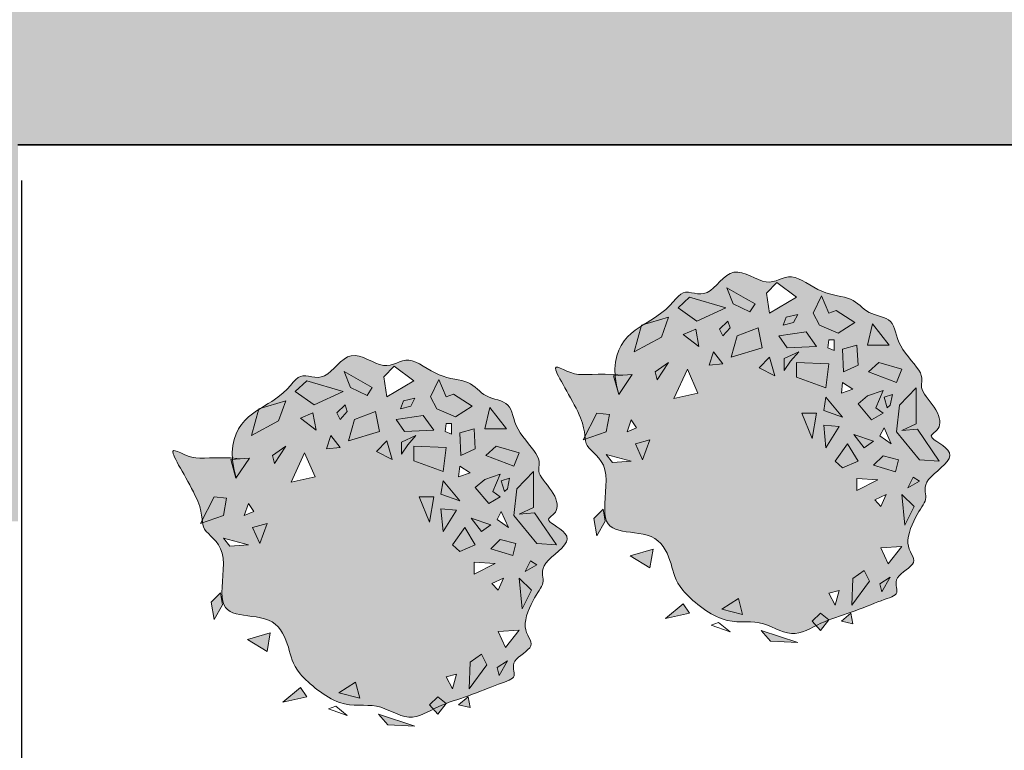
# Model space of a CAD drawing. Units: metres. Extents: x 4298.5 to 4325.2, y 2075 to 2095.8.
# Tile 30 of 35: x 4320.314 to 4321.936, y 2083.561 to 2084.765. Entities that reach past the tile are written whole.
import ezdxf

# ---------------------------------------------------------------- set-up
doc = ezdxf.new("R2010")
doc.units = ezdxf.units.M
for name, color, linetype, lineweight in [('A-ANNO-DIMS', 2, 'Continuous', 18), ('A-WALL', 7, 'Continuous', 35), ('A-WALL-PATT', 252, 'Continuous', 13), ('L-PLNT', 94, 'Continuous', 13)]:
    doc.layers.add(name, color=color, linetype=linetype, lineweight=lineweight)
doc.layers.add('L-PLNT-PATT', color=116, linetype='Continuous', lineweight=13, true_color=0x13823e)
doc.styles.get("Standard").update_dxf_attribs({"font": 'arial.ttf'})
doc.dimstyles.get("Standard").update_dxf_attribs({"dimtxt": 0.18, "dimasz": 0.18, "dimexe": 0.18, "dimexo": 0.0625, "dimgap": 0.09, "dimtad": 0, "dimtih": 1, "dimtoh": 1, "dimdec": 4, "dimzin": 0, "dimdsep": 46, "dimtxsty": 'Standard', "dimcen": 0.09, "dimadec": 0, "dimazin": 0, "dimtfac": 1, "dimtdec": 4, "dimtofl": 0, "dimtmove": 0, "dimatfit": 3, "dimfxl": 1, "dimtolj": 1, "dimtzin": 0, "dimarcsym": 0})

# ---------------------------------------------------------------- blocks, each defined once
blk = doc.blocks.new('*U9')
for points in [[(-2.003, 11.656), (-1.598, 10.618), (-0.518, 10.099), (-0.181, 10.618), (-0.788, 10.964)], [(1.237, 12.003), (0.562, 11.31), (0.764, 10.013), (2.519, 11.051)], [(-4.432, 11.051), (-5.175, 10.359), (-3.96, 9.493), (-2.07, 10.359)], [(4.139, 11.137), (3.599, 10.013), (4.004, 9.234), (5.218, 8.715), (6.298, 9.407), (5.083, 10.186), (4.611, 10.013)], [(-5.782, 9.753), (-7.537, 9.234), (-8.009, 7.504), (-6.255, 8.455)], [(2.586, 9.926), (1.844, 9.753), (1.642, 9.234), (2.316, 9.407)], [(-4.837, 8.628), (-3.825, 7.85), (-4.027, 8.974)], [(-1.935, 9.493), (-2.475, 8.974), (-2.273, 8.542), (-1.8, 9.061)], [(0.022, 9.061), (-1.328, 8.542), (-1.733, 7.157), (0.292, 7.763)], [(7.446, 9.32), (7.108, 7.936), (8.525, 7.936)], [(1.372, 8.542), (3.126, 8.801), (3.801, 7.85), (1.912, 7.763)], [(4.611, 8.282), (4.544, 7.763), (4.949, 7.59), (4.949, 8.282)], [(6.433, 7.936), (5.488, 7.676), (5.556, 6.206), (6.501, 6.638)], [(-2.88, 7.504), (-3.15, 6.638), (-2.273, 6.725)], [(0.764, 7.157), (0.089, 6.465), (1.102, 5.946)], [(1.709, 6.292), (1.709, 7.071), (2.654, 7.504), (2.114, 6.898)], [(-5.782, 6.811), (-6.659, 6.206), (-6.524, 5.687)], [(2.519, 6.811), (2.519, 5.86), (4.409, 5.167), (4.611, 6.725)], [(7.851, 6.811), (7.176, 6.206), (8.998, 5.514), (9.335, 6.379)], [(-8.144, 6.033), (-9.359, 5.946), (-9.022, 4.735)], [(-4.567, 6.379), (-5.445, 4.475), (-3.892, 4.821)], [(5.488, 5.514), (5.421, 4.821), (6.163, 5.081)], [(10.28, 5.167), (9.2, 4.043), (8.998, 2.312), (10.482, 0.495), (11.765, 0.409), (10.348, 2.485), (9.335, 2.399), (10.28, 2.831)], [(4.409, 4.562), (4.274, 3.697), (5.488, 3.264)], [(8.12, 4.994), (7.108, 4.648), (6.501, 4.129), (7.378, 3.091), (8.12, 3.524), (7.648, 3.87)], [(8.728, 4.735), (8.188, 4.562), (8.39, 3.87), (8.593, 4.043)], [(-11.316, 1.793), (-9.831, 2.312), (-9.629, 3.437), (-10.439, 3.524)], [(3.531, 1.88), (2.856, 3.524), (3.801, 3.524)], [(-8.212, 3.091), (-8.482, 2.312), (-7.874, 2.572)], [(4.274, 2.745), (5.286, 2.658), (4.409, 1.274)], [(8.188, 2.572), (7.918, 2.053), (8.66, 1.534)], [(7.513, 1.707), (6.906, 1.274), (6.231, 2.139)], [(-6.997, 1.793), (-7.942, 1.534), (-7.469, 0.495)], [(5.826, 1.534), (5.016, 0.409), (5.488, -0.024), (6.501, 0.409)], [(-8.212, 0.409), (-9.426, 0.322), (-9.831, 0.841)], [(8.12, 0.755), (7.513, 0.149), (8.93, -0.283), (9.133, 0.495)], [(10.078, -0.629), (9.74, -1.322), (10.482, -0.889)], [(7.783, -0.803), (6.433, -1.495), (6.433, -0.716)], [(8.323, -1.754), (7.985, -2.533), (7.581, -2.1)], [(9.335, -1.754), (9.538, -3.744), (10.145, -2.533)], [(-10.034, -2.706), (-10.641, -3.312), (-10.439, -4.436), (-9.899, -3.485)], [(-8.279, -5.734), (-6.794, -5.302), (-6.997, -6.513)], [(9.335, -5.129), (8.458, -6.253), (7.985, -5.215)], [(6.096, -8.935), (6.163, -7.205), (6.906, -6.686), (7.243, -7.378)], [(8.053, -8.07), (8.593, -7.118), (7.918, -7.551)], [(5.286, -7.984), (4.611, -8.157), (5.016, -8.935)], [(-4.837, -8.849), (-4.432, -9.454), (-5.985, -9.801)], [(-2.34, -9.195), (-1.26, -8.503), (-0.99, -9.541)], [(4.071, -9.454), (3.531, -9.974), (4.071, -10.579), (4.611, -9.887)], [(6.028, -9.454), (5.421, -9.974), (6.163, -10.147)], [(-2.543, -10.06), (-3.015, -10.233), (-1.8, -10.666)], [(0.224, -10.579), (0.832, -11.272), (2.586, -11.358)]]:
    blk.add_lwpolyline(points, close=True)
blk = doc.blocks.new('*D47')
at = {"layer": 'A-ANNO-DIMS', "color": 0, "lineweight": -2, "transparency": 16777216}
for p, q in [((4300.4306, 2084.4956), (4300.4306, 2074.9896)), ((4322.8106, 2084.4956), (4322.8106, 2074.9896)), ((4300.6106, 2075.1696), (4311.2252, 2075.1696)), ((4322.6306, 2075.1696), (4312.016, 2075.1696))]:
    blk.add_line(p, q, dxfattribs=at)
at = {"layer": 'A-ANNO-DIMS', "color": 0, "transparency": 16777216}
for points in [[(4300.6106, 2075.1996), (4300.6106, 2075.1396), (4300.4306, 2075.1696)], [(4322.6306, 2075.1996), (4322.6306, 2075.1396), (4322.8106, 2075.1696)]]:
    blk.add_solid(points, dxfattribs=at)
at = {"layer": 'Defpoints', "color": 0, "transparency": 16777216}
for p in [(4300.4306, 2084.5581), (4322.8106, 2084.5581), (4322.8106, 2075.1696)]:
    blk.add_point(p, dxfattribs=at)
at = {"layer": 'A-ANNO-DIMS', "color": 0, "transparency": 16777216, "insert": (4311.6206, 2075.1696), "char_height": 0.18, "attachment_point": 5}
blk.add_mtext('\\A1;22.38', dxfattribs=at)
blk = doc.blocks.new('*D48')
at = {"layer": 'A-ANNO-DIMS', "color": 0, "lineweight": -2, "transparency": 16777216}
for p, q in [((4310.1831, 2094.4781), (4324.7671, 2094.4781)), ((4324.5871, 2094.2981), (4324.5871, 2085.585)), ((4324.5871, 2076.5081), (4324.5871, 2085.2212)), ((4316.8731, 2076.3281), (4324.7671, 2076.3281))]:
    blk.add_line(p, q, dxfattribs=at)
at = {"layer": 'A-ANNO-DIMS', "color": 0, "transparency": 16777216}
for points in [[(4324.5571, 2094.2981), (4324.6171, 2094.2981), (4324.5871, 2094.4781)], [(4324.5571, 2076.5081), (4324.6171, 2076.5081), (4324.5871, 2076.3281)]]:
    blk.add_solid(points, dxfattribs=at)
at = {"layer": 'Defpoints', "color": 0, "transparency": 16777216}
for p in [(4310.1206, 2094.4781), (4316.8106, 2076.3281), (4324.5871, 2076.3281)]:
    blk.add_point(p, dxfattribs=at)
at = {"layer": 'A-ANNO-DIMS', "color": 0, "transparency": 16777216, "insert": (4324.5871, 2085.4031), "char_height": 0.18, "attachment_point": 5}
blk.add_mtext('\\A1;18.15', dxfattribs=at)
blk = doc.blocks.new('*D55')
at = {"layer": 'A-ANNO-DIMS', "color": 0, "lineweight": -2, "transparency": 16777216}
for p, q in [((4320.3167, 2084.4996), (4320.3167, 2074.9896)), ((4322.8106, 2084.4956), (4322.8106, 2074.9896)), ((4320.4967, 2075.1696), (4321.1688, 2075.1696)), ((4322.6306, 2075.1696), (4321.9585, 2075.1696))]:
    blk.add_line(p, q, dxfattribs=at)
at = {"layer": 'A-ANNO-DIMS', "color": 0, "transparency": 16777216}
for points in [[(4320.4967, 2075.1996), (4320.4967, 2075.1396), (4320.3167, 2075.1696)], [(4322.6306, 2075.1996), (4322.6306, 2075.1396), (4322.8106, 2075.1696)]]:
    blk.add_solid(points, dxfattribs=at)
at = {"layer": 'Defpoints', "color": 0, "transparency": 16777216}
for p in [(4320.3167, 2084.5621), (4322.8106, 2084.5581), (4322.8106, 2075.1696)]:
    blk.add_point(p, dxfattribs=at)
at = {"layer": 'A-ANNO-DIMS', "color": 0, "transparency": 16777216, "insert": (4321.5636, 2075.1696), "char_height": 0.18, "attachment_point": 5}
blk.add_mtext('\\A1;2.494', dxfattribs=at)

msp = doc.modelspace()

# ---------------------------------------------------------------- hatches: boundary and pattern name
at = {"layer": 'A-WALL-PATT'}
h = msp.add_hatch(color=256, dxfattribs=at)
h.dxf.hatch_style = 1
h.paths.add_polyline_path([(4308.7606, 2094.4781), (4308.1606, 2094.4781), (4307.4606, 2094.4781), (4307.4606, 2094.2481), (4308.2706, 2094.2481), (4308.2706, 2094.1281), (4308.3906, 2094.1281), (4308.3906, 2094.2481), (4308.7606, 2094.2481)])
h.paths.add_polyline_path([(4310.1206, 2094.4781), (4309.5206, 2094.4781), (4309.5206, 2094.2481), (4309.8906, 2094.2481), (4309.8906, 2092.2481), (4308.3906, 2092.2481), (4308.3906, 2093.4281), (4308.2706, 2093.4281), (4308.2706, 2092.0181), (4309.8906, 2092.0181), (4309.8906, 2087.0181), (4309.7706, 2087.0181), (4309.7706, 2086.7881), (4309.8906, 2086.7881), (4311.9406, 2086.7881), (4311.9406, 2087.0181), (4310.1206, 2087.0181), (4310.1206, 2089.0181), (4310.2406, 2089.0181), (4310.2406, 2089.1381), (4310.1206, 2089.1381), (4310.1206, 2092.0181), (4310.3078, 2092.0181), (4310.3078, 2092.2481), (4310.1206, 2092.2481)])
h.paths.add_polyline_path([(4311.7406, 2092.2481), (4311.0678, 2092.2481), (4311.0678, 2092.0181), (4311.7406, 2092.0181)], flags=17)
h.paths.add_polyline_path([(4313.1733, 2092.2481), (4312.5006, 2092.2481), (4312.5006, 2092.0181), (4313.1733, 2092.0181)])
h.paths.add_polyline_path([(4314.5378, 2092.2481), (4314.1206, 2092.2481), (4313.9333, 2092.2481), (4313.9333, 2092.0181), (4314.1206, 2092.0181), (4314.1206, 2087.0181), (4314.0006, 2087.0181), (4314.0006, 2086.7881), (4314.1206, 2086.7881), (4315.5718, 2086.7881), (4315.5718, 2087.0181), (4314.3506, 2087.0181), (4314.3506, 2092.0181), (4314.5378, 2092.0181)])
h.paths.add_polyline_path([(4315.9706, 2092.2481), (4315.2978, 2092.2481), (4315.2978, 2092.0181), (4315.9706, 2092.0181)])
h.paths.add_polyline_path([(4317.4033, 2092.2481), (4316.7306, 2092.2481), (4316.7306, 2092.0181), (4317.4033, 2092.0181)])
h.paths.add_polyline_path([(4318.9506, 2092.2481), (4318.3506, 2092.2481), (4318.1633, 2092.2481), (4318.1633, 2092.0181), (4318.3506, 2092.0181), (4318.3506, 2091.8981), (4318.5806, 2091.8981), (4318.5806, 2092.0181), (4318.9506, 2092.0181)])
h.paths.add_polyline_path([(4321.0106, 2092.2481), (4319.7106, 2092.2481), (4319.7106, 2092.0181), (4320.0806, 2092.0181), (4320.0806, 2090.0181), (4318.5806, 2090.0181), (4318.5806, 2091.1981), (4318.3506, 2091.1981), (4318.3506, 2090.0181), (4318.3506, 2087.0181), (4318.2306, 2087.0181), (4318.2306, 2086.7881), (4318.3506, 2086.7881), (4318.3506, 2086.3081), (4318.5806, 2086.3081), (4318.5806, 2089.7881), (4321.7806, 2089.7881), (4321.7806, 2090.0181), (4320.2006, 2090.0181), (4320.2006, 2092.0181), (4321.0106, 2092.0181)])
h.paths.add_polyline_path([(4322.8106, 2092.2481), (4321.7706, 2092.2481), (4321.7706, 2092.0181), (4322.5806, 2092.0181), (4322.5806, 2091.2831), (4322.8106, 2091.2831)])
h.paths.add_polyline_path([(4322.8106, 2090.5231), (4322.5806, 2090.5231), (4322.5806, 2089.7881), (4322.5806, 2089.5254), (4322.8106, 2089.5254), (4322.8106, 2090.0181)])
h.paths.add_polyline_path([(4322.8106, 2088.7654), (4322.5806, 2088.7654), (4322.5806, 2087.6681), (4322.8106, 2087.6681)])
h.paths.add_polyline_path([(4322.8106, 2086.9081), (4322.5806, 2086.9081), (4322.5806, 2085.8107), (4322.8106, 2085.8107)])
h.paths.add_polyline_path([(4322.8106, 2085.0507), (4322.5806, 2085.0507), (4322.5806, 2084.7881), (4318.5806, 2084.7881), (4318.5806, 2085.0581), (4318.5806, 2085.4081), (4318.3506, 2085.4081), (4318.3506, 2084.5581), (4318.3506, 2080.8581), (4318.4706, 2080.8581), (4318.4706, 2082.3281), (4319.2606, 2082.3281), (4319.2606, 2082.5581), (4318.5806, 2082.5581), (4318.5806, 2084.5581), (4320.0806, 2084.5581), (4320.0806, 2083.9381), (4320.3106, 2083.9381), (4320.3106, 2084.5581), (4322.8106, 2084.5581)])
h.paths.add_polyline_path([(4320.3106, 2083.1781), (4320.0806, 2083.1781), (4320.0806, 2082.5581), (4319.9606, 2082.5581), (4319.9606, 2082.3281), (4320.0806, 2082.3281), (4320.0806, 2081.5731), (4320.3106, 2081.5731)], flags=17)
h.paths.add_polyline_path([(4320.3106, 2080.8131), (4320.0806, 2080.8131), (4320.0806, 2080.0581), (4318.4286, 2080.0581), (4318.4286, 2079.8281), (4320.3106, 2079.8281)])
h.paths.add_polyline_path([(4317.3506, 2085.2881), (4316.5718, 2085.2881), (4316.5718, 2085.0581), (4317.3506, 2085.0581)])
h.paths.add_polyline_path([(4315.5718, 2085.2881), (4314.8434, 2085.2881), (4314.8434, 2085.0581), (4315.5718, 2085.0581)])
h.paths.add_polyline_path([(4313.8434, 2085.2881), (4312.9406, 2085.2881), (4312.9406, 2085.0581), (4313.8434, 2085.0581)])
h.paths.add_polyline_path([(4311.9406, 2085.2881), (4311.4406, 2085.2881), (4311.4406, 2085.0581), (4311.9406, 2085.0581)])
h.paths.add_polyline_path([(4317.3306, 2087.0181), (4316.5718, 2087.0181), (4316.5718, 2086.7881), (4317.3306, 2086.7881)])
h.paths.add_polyline_path([(4313.1006, 2089.1381), (4311.1406, 2089.1381), (4311.1406, 2089.0181), (4312.9806, 2089.0181), (4312.9806, 2087.0181), (4312.9406, 2087.0181), (4312.9406, 2086.7881), (4313.1006, 2086.7881), (4313.1006, 2087.0181)])
h.paths.add_polyline_path([(4307.5515, 2087.0181), (4305.8906, 2087.0181), (4305.8906, 2092.2481), (4305.8906, 2094.2481), (4306.7006, 2094.2481), (4306.7006, 2094.4781), (4305.6606, 2094.4781), (4305.6606, 2092.2481), (4305.2906, 2092.2481), (4305.2906, 2092.0181), (4305.6606, 2092.0181), (4305.6606, 2090.0181), (4304.1606, 2090.0181), (4304.1606, 2091.1981), (4304.0406, 2091.1981), (4304.0406, 2089.9081), (4301.5606, 2089.9081), (4301.5606, 2089.7881), (4304.0406, 2089.7881), (4305.6606, 2089.7881), (4305.6606, 2086.6381), (4305.8906, 2086.6381), (4305.8906, 2086.7881), (4307.5515, 2086.7881)])
h.paths.add_polyline_path([(4307.5515, 2085.2881), (4305.8906, 2085.2881), (4305.8906, 2085.4381), (4305.6606, 2085.4381), (4305.6606, 2084.7881), (4305.2906, 2084.7881), (4305.2906, 2084.5581), (4305.6606, 2084.5581), (4305.6606, 2084.02), (4305.8906, 2084.02), (4305.8906, 2084.5581), (4305.8906, 2085.0581), (4307.5515, 2085.0581)])
h.paths.add_polyline_path([(4310.2406, 2085.2881), (4308.5515, 2085.2881), (4308.5515, 2085.0581), (4310.2406, 2085.0581)])
h.paths.add_polyline_path([(4317.4286, 2080.0581), (4316.5718, 2080.0581), (4316.5718, 2079.8281), (4317.4286, 2079.8281)])
h.paths.add_polyline_path([(4315.5718, 2080.0581), (4314.8434, 2080.0581), (4314.8434, 2079.8281), (4315.5718, 2079.8281)])
h.paths.add_polyline_path([(4313.8434, 2080.0581), (4312.9406, 2080.0581), (4312.9406, 2079.8281), (4313.8434, 2079.8281)])
h.paths.add_polyline_path([(4311.9406, 2080.0581), (4311.4406, 2080.0581), (4311.4406, 2079.8281), (4311.9406, 2079.8281)])
h.paths.add_polyline_path([(4310.2406, 2080.0581), (4310.1206, 2080.0581), (4310.1206, 2084.0381), (4309.8906, 2084.0381), (4309.8906, 2080.0581), (4309.1606, 2080.0581), (4309.1606, 2079.8281), (4310.2406, 2079.8281)])
h.paths.add_polyline_path([(4308.1606, 2080.0581), (4307.5106, 2080.0581), (4307.5106, 2080.1781), (4307.3906, 2080.1781), (4307.3906, 2080.0581), (4305.8906, 2080.0581), (4305.8906, 2080.567), (4305.6606, 2080.567), (4305.6606, 2079.8281), (4308.1606, 2079.8281)])
h.paths.add_polyline_path([(4307.5106, 2081.9381), (4309.0906, 2081.9381), (4309.0906, 2082.0581), (4305.8906, 2082.0581), (4305.8906, 2083.26), (4305.6606, 2083.26), (4305.6606, 2081.327), (4305.8906, 2081.327), (4305.8906, 2081.9381), (4307.3906, 2081.9381), (4307.3906, 2080.8781), (4307.5106, 2080.8781)])
h.paths.add_polyline_path([(4304.5306, 2084.7881), (4302.7306, 2084.7881), (4302.7306, 2084.5581), (4304.5306, 2084.5581)])
h.paths.add_polyline_path([(4301.9706, 2084.7881), (4300.6606, 2084.7881), (4300.6606, 2085.0249), (4300.4306, 2085.0249), (4300.4306, 2084.5581), (4301.9706, 2084.5581)])
h.paths.add_polyline_path([(4300.6606, 2086.8843), (4300.4306, 2086.8843), (4300.4306, 2085.7849), (4300.6606, 2085.7849)])
h.paths.add_polyline_path([(4300.6606, 2089.1618), (4300.4306, 2089.1618), (4300.4306, 2087.6443), (4300.6606, 2087.6443)])
h.paths.add_polyline_path([(4300.6606, 2091.0212), (4300.4306, 2091.0212), (4300.4306, 2089.9218), (4300.6606, 2089.9218)])
h.paths.add_polyline_path([(4300.6606, 2092.0181), (4301.9706, 2092.0181), (4301.9706, 2092.2481), (4300.4306, 2092.2481), (4300.4306, 2091.7812), (4300.6606, 2091.7812)])
h.paths.add_polyline_path([(4304.5306, 2092.2481), (4302.7306, 2092.2481), (4302.7306, 2092.0181), (4304.0406, 2092.0181), (4304.0406, 2091.8981), (4304.1606, 2091.8981), (4304.1606, 2092.0181), (4304.5306, 2092.0181)], flags=17)
at = {"layer": 'L-PLNT-PATT'}
h = msp.add_hatch(color=256, dxfattribs=at)
h.dxf.hatch_style = 1
edge = h.paths.add_edge_path()
edge.add_spline(control_points=[(4321.6257, 2083.766), (4321.6282, 2083.7673), (4321.6469, 2083.7766), (4321.6827, 2083.7864), (4321.7372, 2083.8096), (4321.7665, 2083.8173), (4321.7478, 2083.8457), (4321.8004, 2083.8699), (4321.7667, 2083.8962), (4321.7937, 2083.956), (4321.8124, 2083.9754), (4321.7958, 2084.0039), (4321.87, 2084.0488), (4321.8001, 2084.0784), (4321.8328, 2084.086), (4321.8288, 2084.1211), (4321.7907, 2084.1577), (4321.8093, 2084.1771), (4321.7562, 2084.2281), (4321.7562, 2084.2741), (4321.7083, 2084.2775), (4321.6879, 2084.3094), (4321.6347, 2084.3094), (4321.5824, 2084.3547), (4321.5476, 2084.3176), (4321.4869, 2084.3685), (4321.447, 2084.2984), (4321.4024, 2084.3284), (4321.3881, 2084.289), (4321.3478, 2084.266), (4321.3414, 2084.262)], knot_values=[0.818571, 0.818571, 0.818571, 0.818571, 0.97924, 1.97924, 2.97924, 3.97924, 4.97924, 5.97924, 6.97924, 7.97924, 8.97924, 9.97924, 10.97924, 11.97924, 12.97924, 13.97924, 14.97924, 15.97924, 16.97924, 17.97924, 18.97924, 19.97924, 20.97924, 21.97924, 22.97924, 23.97924, 24.97924, 25.97924, 26.97924, 27.16067, 27.16067, 27.16067, 27.16067], degree=3, periodic=0)
edge.add_line((4321.3414, 2084.262), (4321.3827, 2084.2742))
edge.add_line((4321.3827, 2084.2742), (4321.3707, 2084.2413))
edge.add_line((4321.3707, 2084.2413), (4321.3261, 2084.2171))
edge.add_line((4321.3261, 2084.2171), (4321.3377, 2084.2597))
edge.add_spline(control_points=[(4321.3377, 2084.2597), (4321.3151, 2084.245), (4321.2918, 2084.2241), (4321.2945, 2084.1797)], knot_values=[0.141368, 0.141368, 0.141368, 0.141368, 0.783694, 0.783694, 0.783694, 0.783694], degree=3, periodic=0)
edge.add_spline(control_points=[(4321.2945, 2084.1797), (4321.2985, 2084.1794), (4321.3027, 2084.1791), (4321.3073, 2084.1786)], knot_values=[40.901028, 40.901028, 40.901028, 40.901028, 41, 41, 41, 41], degree=3, periodic=0)
edge.add_line((4321.3073, 2084.1786), (4321.3227, 2084.1797))
edge.add_line((4321.3227, 2084.1797), (4321.3004, 2084.1468))
edge.add_line((4321.3004, 2084.1468), (4321.2918, 2084.1775))
edge.add_line((4321.2918, 2084.1775), (4321.2947, 2084.1777))
edge.add_spline(control_points=[(4321.2947, 2084.1777), (4321.2946, 2084.1784), (4321.2946, 2084.179), (4321.2945, 2084.1797)], knot_values=[0.13204, 0.13204, 0.13204, 0.13204, 0.141368, 0.141368, 0.141368, 0.141368], degree=3, periodic=0)
edge.add_spline(control_points=[(4321.2945, 2084.1797), (4321.2583, 2084.182), (4321.2267, 2084.1722), (4321.1747, 2084.2142), (4321.2418, 2084.1116), (4321.2441, 2084.0848), (4321.2448, 2084.0773)], knot_values=[37.439141, 37.439141, 37.439141, 37.439141, 38.340169, 39.340169, 40.340169, 40.901028, 40.901028, 40.901028, 40.901028], degree=3, periodic=0)
edge.add_line((4321.2448, 2084.0773), (4321.2644, 2084.116))
edge.add_line((4321.2644, 2084.116), (4321.285, 2084.1138))
edge.add_line((4321.285, 2084.1138), (4321.2798, 2084.0852))
edge.add_line((4321.2798, 2084.0852), (4321.2452, 2084.0731))
edge.add_spline(control_points=[(4321.2452, 2084.0731), (4321.2457, 2084.0692), (4321.2488, 2084.0556), (4321.2901, 2084.0347), (4321.2687, 2083.9374), (4321.3009, 2083.9186), (4321.3671, 2083.9186), (4321.3899, 2083.8648), (4321.3934, 2083.8293), (4321.4744, 2083.7633), (4321.5327, 2083.7801), (4321.5831, 2083.7432), (4321.6122, 2083.7591), (4321.6257, 2083.766)], knot_values=[27.16067, 27.16067, 27.16067, 27.16067, 27.490087, 28.490087, 29.490087, 30.490087, 31.490087, 32.490087, 33.490087, 34.490087, 35.490087, 36.490087, 37.329418, 37.329418, 37.329418, 37.329418], degree=3, periodic=0)
edge.add_line((4321.6257, 2083.766), (4321.6192, 2083.7732))
edge.add_line((4321.6192, 2083.7732), (4321.633, 2083.7864))
edge.add_line((4321.633, 2083.7864), (4321.6467, 2083.7754))
h.paths.add_polyline_path([(4321.6021, 2084.116), (4321.6261, 2084.116), (4321.6192, 2084.0743)], flags=16)
h.paths.add_polyline_path([(4321.6381, 2084.0962), (4321.6638, 2084.094), (4321.6415, 2084.0589)], flags=16)
h.paths.add_polyline_path([(4321.4307, 2084.149), (4321.3913, 2084.1402), (4321.4136, 2084.1885)], flags=16)
h.paths.add_polyline_path([(4321.5575, 2084.1775), (4321.5318, 2084.1907), (4321.549, 2084.2083)], flags=16)
h.paths.add_polyline_path([(4321.6381, 2084.1204), (4321.6415, 2084.1424), (4321.6689, 2084.1094)], flags=16)
h.paths.add_polyline_path([(4321.657, 2084.0369), (4321.6775, 2084.0655), (4321.6947, 2084.0369), (4321.6689, 2084.0259)], flags=16)
h.paths.add_polyline_path([(4321.5935, 2084.1753), (4321.5935, 2084.1995), (4321.6467, 2084.1973), (4321.6415, 2084.1577)], flags=16)
h.paths.add_polyline_path([(4321.573, 2084.1863), (4321.573, 2084.2061), (4321.597, 2084.2171), (4321.5833, 2084.2017)], flags=16)
h.paths.add_polyline_path([(4321.4718, 2084.1973), (4321.4495, 2084.1951), (4321.4564, 2084.2171)], flags=16)
h.paths.add_polyline_path([(4321.4855, 2084.2083), (4321.4958, 2084.2435), (4321.5301, 2084.2567), (4321.537, 2084.2237)], flags=16)
h.paths.add_polyline_path([(4321.3518, 2084.072), (4321.3398, 2084.0391), (4321.3278, 2084.0655)], flags=16)
h.paths.add_polyline_path([(4321.6878, 2084.0808), (4321.7204, 2084.0699), (4321.705, 2084.0589)], flags=16)
h.paths.add_polyline_path([(4321.6672, 2084.149), (4321.6689, 2084.1666), (4321.6861, 2084.1556)], flags=16)
h.paths.add_polyline_path([(4321.5781, 2084.2237), (4321.5644, 2084.2435), (4321.609, 2084.25), (4321.6261, 2084.2259)], flags=16)
h.paths.add_polyline_path([(4321.693, 2084.0083), (4321.7272, 2084.0061), (4321.693, 2083.9885)], flags=16)
h.paths.add_polyline_path([(4321.3296, 2084.0918), (4321.3141, 2084.0852), (4321.321, 2084.105)], flags=16)
h.paths.add_polyline_path([(4321.4324, 2084.2259), (4321.4067, 2084.2457), (4321.4273, 2084.2544)], flags=16)
h.paths.add_polyline_path([(4321.3638, 2084.171), (4321.3604, 2084.1841), (4321.3827, 2084.1995)], flags=16)
h.paths.add_polyline_path([(4321.4718, 2084.2435), (4321.4667, 2084.2544), (4321.4804, 2084.2676), (4321.4838, 2084.2567)], flags=16)
h.paths.add_polyline_path([(4321.6947, 2084.1314), (4321.7101, 2084.1446), (4321.7358, 2084.1534), (4321.7238, 2084.1248), (4321.7358, 2084.116), (4321.717, 2084.105)], flags=16)
h.paths.add_polyline_path([(4321.321, 2084.0369), (4321.2901, 2084.0347), (4321.2798, 2084.0479)], flags=16)
h.paths.add_polyline_path([(4321.6707, 2084.1841), (4321.6689, 2084.2215), (4321.693, 2084.2281), (4321.6947, 2084.1951)], flags=16)
h.paths.add_polyline_path([(4321.7204, 2084.0303), (4321.7358, 2084.0457), (4321.7615, 2084.0391), (4321.7564, 2084.0193)], flags=16)
h.paths.add_polyline_path([(4321.645, 2084.2237), (4321.6467, 2084.2369), (4321.6553, 2084.2369), (4321.6553, 2084.2193)], flags=16)
h.paths.add_polyline_path([(4321.5713, 2084.261), (4321.5764, 2084.2742), (4321.5952, 2084.2786), (4321.5884, 2084.2654)], flags=16)
h.paths.add_polyline_path([(4321.7307, 2084.0786), (4321.7375, 2084.0918), (4321.7495, 2084.0655)], flags=16)
h.paths.add_polyline_path([(4321.7221, 2083.9732), (4321.741, 2083.982), (4321.7324, 2083.9622)], flags=16)
h.paths.add_polyline_path([(4321.5164, 2084.283), (4321.489, 2084.2962), (4321.4787, 2084.3226), (4321.5095, 2084.305), (4321.525, 2084.2962)], flags=16)
h.paths.add_polyline_path([(4321.549, 2084.2808), (4321.5438, 2084.3138), (4321.561, 2084.3314), (4321.5935, 2084.3072)], flags=16)
h.paths.add_polyline_path([(4321.429, 2084.2676), (4321.3981, 2084.2896), (4321.417, 2084.3072), (4321.477, 2084.2896)], flags=16)
h.paths.add_polyline_path([(4321.7118, 2084.1841), (4321.729, 2084.1995), (4321.7667, 2084.1885), (4321.7581, 2084.1666)], flags=16)
h.paths.add_polyline_path([(4321.6313, 2084.261), (4321.621, 2084.2808), (4321.6347, 2084.3094), (4321.6467, 2084.2808), (4321.6587, 2084.2852), (4321.6895, 2084.2654), (4321.6621, 2084.2479)], flags=16)
h.paths.add_polyline_path([(4321.7427, 2084.1248), (4321.7375, 2084.1424), (4321.7512, 2084.1468), (4321.7478, 2084.1292)], flags=16)
h.paths.add_polyline_path([(4321.7581, 2084.0852), (4321.7632, 2084.1292), (4321.7907, 2084.1577), (4321.7907, 2084.0984), (4321.7667, 2084.0874), (4321.7924, 2084.0896), (4321.8284, 2084.0369), (4321.7958, 2084.0391)], flags=16)
h.paths.add_polyline_path([(4321.4976, 2083.8105), (4321.5044, 2083.7842), (4321.4701, 2083.793)], flags=16)
h.paths.add_polyline_path([(4321.7101, 2084.2281), (4321.7187, 2084.2632), (4321.7461, 2084.2281)], flags=16)
h.paths.add_polyline_path([(4321.7667, 2083.982), (4321.7872, 2083.9622), (4321.7718, 2083.9314)], flags=16)
h.paths.add_polyline_path([(4321.777, 2083.9929), (4321.7855, 2084.0105), (4321.7958, 2084.0039)], flags=16)
h.paths.add_polyline_path([(4321.6467, 2083.8193), (4321.6638, 2083.8237), (4321.657, 2083.7996)], flags=16)
h.paths.add_polyline_path([(4321.7324, 2083.894), (4321.7667, 2083.8962), (4321.7444, 2083.8677)], flags=16)
h.paths.add_polyline_path([(4321.6861, 2083.8435), (4321.705, 2083.8567), (4321.7135, 2083.8391), (4321.6844, 2083.7996)], flags=16)
h.paths.add_polyline_path([(4321.7307, 2083.8347), (4321.7478, 2083.8457), (4321.7341, 2083.8215)], flags=16)
h = msp.add_hatch(color=256, dxfattribs=at)
h.dxf.hatch_style = 1
h.paths.add_polyline_path([(4321.6415, 2084.1577), (4321.6467, 2084.1973), (4321.5935, 2084.1995), (4321.5935, 2084.1753)])
h.paths.add_polyline_path([(4321.6878, 2084.0808), (4321.705, 2084.0589), (4321.7204, 2084.0699)])
h.paths.add_polyline_path([(4321.6689, 2084.2215), (4321.6707, 2084.1841), (4321.6947, 2084.1951), (4321.693, 2084.2281)])
h.paths.add_polyline_path([(4321.6895, 2084.2654), (4321.6587, 2084.2852), (4321.6467, 2084.2808), (4321.6347, 2084.3094), (4321.621, 2084.2808), (4321.6313, 2084.261), (4321.6621, 2084.2479)])
h.paths.add_polyline_path([(4321.5352, 2083.7578), (4321.5507, 2083.7402), (4321.5952, 2083.738)])
h.paths.add_polyline_path([(4321.5164, 2084.283), (4321.525, 2084.2962), (4321.5095, 2084.305), (4321.4787, 2084.3226), (4321.489, 2084.2962)])
h.paths.add_polyline_path([(4321.417, 2084.3072), (4321.3981, 2084.2896), (4321.429, 2084.2676), (4321.477, 2084.2896)])
h.paths.add_polyline_path([(4321.4958, 2084.2435), (4321.4855, 2084.2083), (4321.537, 2084.2237), (4321.5301, 2084.2567)])
h.paths.add_polyline_path([(4321.4838, 2084.2567), (4321.4804, 2084.2676), (4321.4667, 2084.2544), (4321.4718, 2084.2435)])
h.paths.add_polyline_path([(4321.4564, 2084.2171), (4321.4495, 2084.1951), (4321.4718, 2084.1973)])
h.paths.add_polyline_path([(4321.4324, 2084.2259), (4321.4273, 2084.2544), (4321.4067, 2084.2457)])
h.paths.add_polyline_path([(4321.3381, 2084.261), (4321.3261, 2084.2171), (4321.3707, 2084.2413), (4321.3827, 2084.2742)])
h.paths.add_polyline_path([(4321.3827, 2084.1995), (4321.3604, 2084.1841), (4321.3638, 2084.171)])
h.paths.add_polyline_path([(4321.2918, 2084.1775), (4321.3004, 2084.1468), (4321.3227, 2084.1797)])
h.paths.add_polyline_path([(4321.2421, 2084.072), (4321.2798, 2084.0852), (4321.285, 2084.1138), (4321.2644, 2084.116)])
h.paths.add_polyline_path([(4321.3518, 2084.072), (4321.3278, 2084.0655), (4321.3398, 2084.0391)])
h.paths.add_polyline_path([(4321.2781, 2083.938), (4321.2747, 2083.9578), (4321.2593, 2083.9424), (4321.2644, 2083.9138)])
h.paths.add_polyline_path([(4321.357, 2083.8918), (4321.3193, 2083.8809), (4321.3518, 2083.8611)])
h.paths.add_polyline_path([(4321.3775, 2083.7776), (4321.417, 2083.7864), (4321.4067, 2083.8017)])
h.paths.add_polyline_path([(4321.4976, 2083.8105), (4321.4701, 2083.793), (4321.5044, 2083.7842)])
h.paths.add_polyline_path([(4321.633, 2083.7864), (4321.6192, 2083.7732), (4321.633, 2083.7578), (4321.6467, 2083.7754)])
h.paths.add_polyline_path([(4321.7135, 2083.8391), (4321.705, 2083.8567), (4321.6861, 2083.8435), (4321.6844, 2083.7996)])
h.paths.add_polyline_path([(4321.6827, 2083.7864), (4321.6672, 2083.7732), (4321.6861, 2083.7688)])
h.paths.add_polyline_path([(4321.7307, 2083.8347), (4321.7341, 2083.8215), (4321.7478, 2083.8457)])
h.paths.add_polyline_path([(4321.7718, 2083.9314), (4321.7872, 2083.9622), (4321.7667, 2083.982)])
h.paths.add_polyline_path([(4321.657, 2084.0369), (4321.6689, 2084.0259), (4321.6947, 2084.0369), (4321.6775, 2084.0655)])
h.paths.add_polyline_path([(4321.7958, 2084.0391), (4321.8284, 2084.0369), (4321.7924, 2084.0896), (4321.7667, 2084.0874), (4321.7907, 2084.0984), (4321.7907, 2084.1577), (4321.7632, 2084.1292), (4321.7581, 2084.0852)])
h.paths.add_polyline_path([(4321.7358, 2084.0457), (4321.7204, 2084.0303), (4321.7564, 2084.0193), (4321.7615, 2084.0391)])
h.paths.add_polyline_path([(4321.7958, 2084.0039), (4321.7855, 2084.0105), (4321.777, 2083.9929)])
h.paths.add_polyline_path([(4321.7358, 2084.1534), (4321.7101, 2084.1446), (4321.6947, 2084.1314), (4321.717, 2084.105), (4321.7358, 2084.116), (4321.7238, 2084.1248)])
h.paths.add_polyline_path([(4321.7375, 2084.1424), (4321.7427, 2084.1248), (4321.7478, 2084.1292), (4321.7512, 2084.1468)])
h.paths.add_polyline_path([(4321.7581, 2084.1666), (4321.7667, 2084.1885), (4321.729, 2084.1995), (4321.7118, 2084.1841)])
h.paths.add_polyline_path([(4321.6689, 2084.1094), (4321.6415, 2084.1424), (4321.6381, 2084.1204)])
h.paths.add_polyline_path([(4321.6261, 2084.116), (4321.6021, 2084.116), (4321.6192, 2084.0743)])
h.paths.add_polyline_path([(4321.6638, 2084.094), (4321.6381, 2084.0962), (4321.6415, 2084.0589)])
h.paths.add_polyline_path([(4321.6261, 2084.2259), (4321.609, 2084.25), (4321.5644, 2084.2435), (4321.5781, 2084.2237)])
h.paths.add_polyline_path([(4321.5833, 2084.2017), (4321.597, 2084.2171), (4321.573, 2084.2061), (4321.573, 2084.1863)])
h.paths.add_polyline_path([(4321.549, 2084.2083), (4321.5318, 2084.1907), (4321.5575, 2084.1775)])
h.paths.add_polyline_path([(4321.5884, 2084.2654), (4321.5952, 2084.2786), (4321.5764, 2084.2742), (4321.5713, 2084.261)])
h.paths.add_polyline_path([(4321.7187, 2084.2632), (4321.7101, 2084.2281), (4321.7461, 2084.2281)])
h = msp.add_hatch(color=256, dxfattribs=at)
h.dxf.hatch_style = 1
edge = h.paths.add_edge_path()
edge.add_spline(control_points=[(4320.9952, 2083.6284), (4320.9978, 2083.6297), (4321.0164, 2083.639), (4321.0522, 2083.6488), (4321.1068, 2083.672), (4321.1361, 2083.6797), (4321.1174, 2083.7081), (4321.17, 2083.7323), (4321.1362, 2083.7586), (4321.1633, 2083.8184), (4321.182, 2083.8378), (4321.1654, 2083.8663), (4321.2396, 2083.9112), (4321.1696, 2083.9408), (4321.2023, 2083.9484), (4321.1983, 2083.9835), (4321.1602, 2084.0202), (4321.1788, 2084.0395), (4321.1258, 2084.0905), (4321.1258, 2084.1365), (4321.0779, 2084.1399), (4321.0575, 2084.1718), (4321.0043, 2084.1718), (4320.9519, 2084.2171), (4320.9171, 2084.18), (4320.8565, 2084.2309), (4320.8165, 2084.1608), (4320.772, 2084.1908), (4320.7576, 2084.1514), (4320.7173, 2084.1284), (4320.711, 2084.1244)], knot_values=[0.818571, 0.818571, 0.818571, 0.818571, 0.97924, 1.97924, 2.97924, 3.97924, 4.97924, 5.97924, 6.97924, 7.97924, 8.97924, 9.97924, 10.97924, 11.97924, 12.97924, 13.97924, 14.97924, 15.97924, 16.97924, 17.97924, 18.97924, 19.97924, 20.97924, 21.97924, 22.97924, 23.97924, 24.97924, 25.97924, 26.97924, 27.16067, 27.16067, 27.16067, 27.16067], degree=3, periodic=0)
edge.add_line((4320.711, 2084.1244), (4320.7523, 2084.1366))
edge.add_line((4320.7523, 2084.1366), (4320.7402, 2084.1037))
edge.add_line((4320.7402, 2084.1037), (4320.6957, 2084.0795))
edge.add_line((4320.6957, 2084.0795), (4320.7073, 2084.1221))
edge.add_spline(control_points=[(4320.7073, 2084.1221), (4320.6847, 2084.1074), (4320.6614, 2084.0865), (4320.6641, 2084.0421)], knot_values=[0.141368, 0.141368, 0.141368, 0.141368, 0.783694, 0.783694, 0.783694, 0.783694], degree=3, periodic=0)
edge.add_spline(control_points=[(4320.6641, 2084.0421), (4320.6681, 2084.0418), (4320.6723, 2084.0415), (4320.6768, 2084.041)], knot_values=[40.901028, 40.901028, 40.901028, 40.901028, 41, 41, 41, 41], degree=3, periodic=0)
edge.add_line((4320.6768, 2084.041), (4320.6923, 2084.0421))
edge.add_line((4320.6923, 2084.0421), (4320.67, 2084.0092))
edge.add_line((4320.67, 2084.0092), (4320.6614, 2084.0399))
edge.add_line((4320.6614, 2084.0399), (4320.6642, 2084.0401))
edge.add_spline(control_points=[(4320.6642, 2084.0401), (4320.6642, 2084.0408), (4320.6641, 2084.0414), (4320.6641, 2084.0421)], knot_values=[0.13204, 0.13204, 0.13204, 0.13204, 0.141368, 0.141368, 0.141368, 0.141368], degree=3, periodic=0)
edge.add_spline(control_points=[(4320.6641, 2084.0421), (4320.6279, 2084.0444), (4320.5963, 2084.0346), (4320.5443, 2084.0766), (4320.6113, 2083.974), (4320.6137, 2083.9472), (4320.6143, 2083.9397)], knot_values=[37.439141, 37.439141, 37.439141, 37.439141, 38.340169, 39.340169, 40.340169, 40.901028, 40.901028, 40.901028, 40.901028], degree=3, periodic=0)
edge.add_line((4320.6143, 2083.9397), (4320.634, 2083.9784))
edge.add_line((4320.634, 2083.9784), (4320.6545, 2083.9762))
edge.add_line((4320.6545, 2083.9762), (4320.6494, 2083.9476))
edge.add_line((4320.6494, 2083.9476), (4320.6148, 2083.9355))
edge.add_spline(control_points=[(4320.6148, 2083.9355), (4320.6153, 2083.9316), (4320.6183, 2083.918), (4320.6597, 2083.8971), (4320.6382, 2083.7998), (4320.6705, 2083.781), (4320.7367, 2083.781), (4320.7595, 2083.7272), (4320.763, 2083.6918), (4320.844, 2083.6257), (4320.9023, 2083.6425), (4320.9526, 2083.6056), (4320.9818, 2083.6215), (4320.9952, 2083.6284)], knot_values=[27.16067, 27.16067, 27.16067, 27.16067, 27.490087, 28.490087, 29.490087, 30.490087, 31.490087, 32.490087, 33.490087, 34.490087, 35.490087, 36.490087, 37.329418, 37.329418, 37.329418, 37.329418], degree=3, periodic=0)
edge.add_line((4320.9952, 2083.6284), (4320.9888, 2083.6356))
edge.add_line((4320.9888, 2083.6356), (4321.0025, 2083.6488))
edge.add_line((4321.0025, 2083.6488), (4321.0163, 2083.6378))
h.paths.add_polyline_path([(4320.9717, 2083.9784), (4320.9957, 2083.9784), (4320.9888, 2083.9367)], flags=16)
h.paths.add_polyline_path([(4321.0077, 2083.9586), (4321.0334, 2083.9564), (4321.0111, 2083.9213)], flags=16)
h.paths.add_polyline_path([(4320.8003, 2084.0114), (4320.7608, 2084.0026), (4320.7831, 2084.0509)], flags=16)
h.paths.add_polyline_path([(4320.9271, 2084.0399), (4320.9014, 2084.0531), (4320.9185, 2084.0707)], flags=16)
h.paths.add_polyline_path([(4321.0077, 2083.9828), (4321.0111, 2084.0048), (4321.0385, 2083.9718)], flags=16)
h.paths.add_polyline_path([(4321.0265, 2083.8993), (4321.0471, 2083.9279), (4321.0643, 2083.8993), (4321.0385, 2083.8883)], flags=16)
h.paths.add_polyline_path([(4320.9631, 2084.0378), (4320.9631, 2084.0619), (4321.0162, 2084.0597), (4321.0111, 2084.0202)], flags=16)
h.paths.add_polyline_path([(4320.9425, 2084.0487), (4320.9425, 2084.0685), (4320.9665, 2084.0795), (4320.9528, 2084.0641)], flags=16)
h.paths.add_polyline_path([(4320.8414, 2084.0597), (4320.8191, 2084.0575), (4320.826, 2084.0795)], flags=16)
h.paths.add_polyline_path([(4320.8551, 2084.0707), (4320.8654, 2084.1059), (4320.8997, 2084.1191), (4320.9065, 2084.0861)], flags=16)
h.paths.add_polyline_path([(4320.7214, 2083.9345), (4320.7094, 2083.9015), (4320.6974, 2083.9279)], flags=16)
h.paths.add_polyline_path([(4321.0574, 2083.9432), (4321.09, 2083.9323), (4321.0745, 2083.9213)], flags=16)
h.paths.add_polyline_path([(4321.0368, 2084.0114), (4321.0385, 2084.029), (4321.0557, 2084.018)], flags=16)
h.paths.add_polyline_path([(4320.9477, 2084.0861), (4320.934, 2084.1059), (4320.9785, 2084.1125), (4320.9957, 2084.0883)], flags=16)
h.paths.add_polyline_path([(4321.0625, 2083.8707), (4321.0968, 2083.8685), (4321.0625, 2083.8509)], flags=16)
h.paths.add_polyline_path([(4320.6991, 2083.9542), (4320.6837, 2083.9476), (4320.6905, 2083.9674)], flags=16)
h.paths.add_polyline_path([(4320.802, 2084.0883), (4320.7763, 2084.1081), (4320.7968, 2084.1169)], flags=16)
h.paths.add_polyline_path([(4320.7334, 2084.0334), (4320.73, 2084.0465), (4320.7523, 2084.0619)], flags=16)
h.paths.add_polyline_path([(4320.8414, 2084.1059), (4320.8363, 2084.1169), (4320.85, 2084.13), (4320.8534, 2084.1191)], flags=16)
h.paths.add_polyline_path([(4321.0643, 2083.9938), (4321.0797, 2084.007), (4321.1054, 2084.0158), (4321.0934, 2083.9872), (4321.1054, 2083.9784), (4321.0865, 2083.9674)], flags=16)
h.paths.add_polyline_path([(4320.6905, 2083.8993), (4320.6597, 2083.8971), (4320.6494, 2083.9103)], flags=16)
h.paths.add_polyline_path([(4321.0402, 2084.0465), (4321.0385, 2084.0839), (4321.0625, 2084.0905), (4321.0643, 2084.0575)], flags=16)
h.paths.add_polyline_path([(4321.09, 2083.8927), (4321.1054, 2083.9081), (4321.1311, 2083.9015), (4321.1259, 2083.8817)], flags=16)
h.paths.add_polyline_path([(4321.0145, 2084.0861), (4321.0162, 2084.0993), (4321.0248, 2084.0993), (4321.0248, 2084.0817)], flags=16)
h.paths.add_polyline_path([(4320.9408, 2084.1235), (4320.946, 2084.1366), (4320.9648, 2084.141), (4320.958, 2084.1278)], flags=16)
h.paths.add_polyline_path([(4321.1002, 2083.9411), (4321.1071, 2083.9542), (4321.1191, 2083.9279)], flags=16)
h.paths.add_polyline_path([(4321.0917, 2083.8356), (4321.1105, 2083.8444), (4321.1019, 2083.8246)], flags=16)
h.paths.add_polyline_path([(4320.886, 2084.1454), (4320.8585, 2084.1586), (4320.8482, 2084.185), (4320.8791, 2084.1674), (4320.8945, 2084.1586)], flags=16)
h.paths.add_polyline_path([(4320.9185, 2084.1432), (4320.9134, 2084.1762), (4320.9305, 2084.1938), (4320.9631, 2084.1696)], flags=16)
h.paths.add_polyline_path([(4320.7985, 2084.13), (4320.7677, 2084.152), (4320.7866, 2084.1696), (4320.8465, 2084.152)], flags=16)
h.paths.add_polyline_path([(4321.0814, 2084.0465), (4321.0985, 2084.0619), (4321.1362, 2084.0509), (4321.1277, 2084.029)], flags=16)
h.paths.add_polyline_path([(4321.0008, 2084.1235), (4320.9905, 2084.1432), (4321.0043, 2084.1718), (4321.0162, 2084.1432), (4321.0282, 2084.1476), (4321.0591, 2084.1278), (4321.0317, 2084.1103)], flags=16)
h.paths.add_polyline_path([(4321.1122, 2083.9872), (4321.1071, 2084.0048), (4321.1208, 2084.0092), (4321.1174, 2083.9916)], flags=16)
h.paths.add_polyline_path([(4321.1277, 2083.9476), (4321.1328, 2083.9916), (4321.1602, 2084.0202), (4321.1602, 2083.9608), (4321.1362, 2083.9498), (4321.162, 2083.952), (4321.198, 2083.8993), (4321.1654, 2083.9015)], flags=16)
h.paths.add_polyline_path([(4320.8671, 2083.6729), (4320.874, 2083.6466), (4320.8397, 2083.6554)], flags=16)
h.paths.add_polyline_path([(4321.0797, 2084.0905), (4321.0883, 2084.1256), (4321.1157, 2084.0905)], flags=16)
h.paths.add_polyline_path([(4321.1362, 2083.8444), (4321.1568, 2083.8246), (4321.1414, 2083.7938)], flags=16)
h.paths.add_polyline_path([(4321.1465, 2083.8553), (4321.1551, 2083.8729), (4321.1654, 2083.8663)], flags=16)
h.paths.add_polyline_path([(4321.0162, 2083.6817), (4321.0334, 2083.6861), (4321.0265, 2083.662)], flags=16)
h.paths.add_polyline_path([(4321.1019, 2083.7565), (4321.1362, 2083.7586), (4321.114, 2083.7301)], flags=16)
h.paths.add_polyline_path([(4321.0557, 2083.7059), (4321.0745, 2083.7191), (4321.0831, 2083.7015), (4321.054, 2083.662)], flags=16)
h.paths.add_polyline_path([(4321.1002, 2083.6971), (4321.1174, 2083.7081), (4321.1037, 2083.6839)], flags=16)
h = msp.add_hatch(color=256, dxfattribs=at)
h.dxf.hatch_style = 1
h.paths.add_polyline_path([(4321.0111, 2084.0202), (4321.0162, 2084.0597), (4320.9631, 2084.0619), (4320.9631, 2084.0378)])
h.paths.add_polyline_path([(4321.0574, 2083.9432), (4321.0745, 2083.9213), (4321.09, 2083.9323)])
h.paths.add_polyline_path([(4321.0385, 2084.0839), (4321.0402, 2084.0465), (4321.0643, 2084.0575), (4321.0625, 2084.0905)])
h.paths.add_polyline_path([(4321.0591, 2084.1278), (4321.0282, 2084.1476), (4321.0162, 2084.1432), (4321.0043, 2084.1718), (4320.9905, 2084.1432), (4321.0008, 2084.1235), (4321.0317, 2084.1103)])
h.paths.add_polyline_path([(4320.9048, 2083.6202), (4320.9203, 2083.6026), (4320.9648, 2083.6004)])
h.paths.add_polyline_path([(4320.886, 2084.1454), (4320.8945, 2084.1586), (4320.8791, 2084.1674), (4320.8482, 2084.185), (4320.8585, 2084.1586)])
h.paths.add_polyline_path([(4320.7866, 2084.1696), (4320.7677, 2084.152), (4320.7985, 2084.13), (4320.8465, 2084.152)])
h.paths.add_polyline_path([(4320.8654, 2084.1059), (4320.8551, 2084.0707), (4320.9065, 2084.0861), (4320.8997, 2084.1191)])
h.paths.add_polyline_path([(4320.8534, 2084.1191), (4320.85, 2084.13), (4320.8363, 2084.1169), (4320.8414, 2084.1059)])
h.paths.add_polyline_path([(4320.826, 2084.0795), (4320.8191, 2084.0575), (4320.8414, 2084.0597)])
h.paths.add_polyline_path([(4320.802, 2084.0883), (4320.7968, 2084.1169), (4320.7763, 2084.1081)])
h.paths.add_polyline_path([(4320.7077, 2084.1235), (4320.6957, 2084.0795), (4320.7402, 2084.1037), (4320.7523, 2084.1366)])
h.paths.add_polyline_path([(4320.7523, 2084.0619), (4320.73, 2084.0465), (4320.7334, 2084.0334)])
h.paths.add_polyline_path([(4320.6614, 2084.0399), (4320.67, 2084.0092), (4320.6923, 2084.0421)])
h.paths.add_polyline_path([(4320.6117, 2083.9345), (4320.6494, 2083.9476), (4320.6545, 2083.9762), (4320.634, 2083.9784)])
h.paths.add_polyline_path([(4320.7214, 2083.9345), (4320.6974, 2083.9279), (4320.7094, 2083.9015)])
h.paths.add_polyline_path([(4320.6477, 2083.8004), (4320.6443, 2083.8202), (4320.6288, 2083.8048), (4320.634, 2083.7762)])
h.paths.add_polyline_path([(4320.7266, 2083.7542), (4320.6888, 2083.7433), (4320.7214, 2083.7235)])
h.paths.add_polyline_path([(4320.7471, 2083.64), (4320.7866, 2083.6488), (4320.7763, 2083.6641)])
h.paths.add_polyline_path([(4320.8671, 2083.6729), (4320.8397, 2083.6554), (4320.874, 2083.6466)])
h.paths.add_polyline_path([(4321.0025, 2083.6488), (4320.9888, 2083.6356), (4321.0025, 2083.6202), (4321.0162, 2083.6378)])
h.paths.add_polyline_path([(4321.0831, 2083.7015), (4321.0745, 2083.7191), (4321.0557, 2083.7059), (4321.054, 2083.662)])
h.paths.add_polyline_path([(4321.0522, 2083.6488), (4321.0368, 2083.6356), (4321.0557, 2083.6312)])
h.paths.add_polyline_path([(4321.1002, 2083.6971), (4321.1037, 2083.6839), (4321.1174, 2083.7081)])
h.paths.add_polyline_path([(4321.1414, 2083.7938), (4321.1568, 2083.8246), (4321.1362, 2083.8444)])
h.paths.add_polyline_path([(4321.0265, 2083.8993), (4321.0385, 2083.8883), (4321.0643, 2083.8993), (4321.0471, 2083.9279)])
h.paths.add_polyline_path([(4321.1654, 2083.9015), (4321.198, 2083.8993), (4321.162, 2083.952), (4321.1362, 2083.9498), (4321.1602, 2083.9608), (4321.1602, 2084.0202), (4321.1328, 2083.9916), (4321.1277, 2083.9476)])
h.paths.add_polyline_path([(4321.1054, 2083.9081), (4321.09, 2083.8927), (4321.1259, 2083.8817), (4321.1311, 2083.9015)])
h.paths.add_polyline_path([(4321.1654, 2083.8663), (4321.1551, 2083.8729), (4321.1465, 2083.8553)])
h.paths.add_polyline_path([(4321.1054, 2084.0158), (4321.0797, 2084.007), (4321.0643, 2083.9938), (4321.0865, 2083.9674), (4321.1054, 2083.9784), (4321.0934, 2083.9872)])
h.paths.add_polyline_path([(4321.1071, 2084.0048), (4321.1122, 2083.9872), (4321.1174, 2083.9916), (4321.1208, 2084.0092)])
h.paths.add_polyline_path([(4321.1277, 2084.029), (4321.1362, 2084.0509), (4321.0985, 2084.0619), (4321.0814, 2084.0465)])
h.paths.add_polyline_path([(4321.0385, 2083.9718), (4321.0111, 2084.0048), (4321.0077, 2083.9828)])
h.paths.add_polyline_path([(4320.9957, 2083.9784), (4320.9717, 2083.9784), (4320.9888, 2083.9367)])
h.paths.add_polyline_path([(4321.0334, 2083.9564), (4321.0077, 2083.9586), (4321.0111, 2083.9213)])
h.paths.add_polyline_path([(4320.9957, 2084.0883), (4320.9785, 2084.1125), (4320.934, 2084.1059), (4320.9477, 2084.0861)])
h.paths.add_polyline_path([(4320.9528, 2084.0641), (4320.9665, 2084.0795), (4320.9425, 2084.0685), (4320.9425, 2084.0487)])
h.paths.add_polyline_path([(4320.9185, 2084.0707), (4320.9014, 2084.0531), (4320.9271, 2084.0399)])
h.paths.add_polyline_path([(4320.958, 2084.1278), (4320.9648, 2084.141), (4320.946, 2084.1366), (4320.9408, 2084.1235)])
h.paths.add_polyline_path([(4321.0883, 2084.1256), (4321.0797, 2084.0905), (4321.1157, 2084.0905)])

# ---------------------------------------------------------------- linework, layer by layer
at = {"layer": 'A-WALL'}
msp.add_line((4322.8106, 2084.5581), (4320.3106, 2084.5581), dxfattribs=at)
at = {"layer": 'L-PLNT'}
for points in [[(4321.3004, 2084.1468), (4321.2763, 2084.2333), (4321.3827, 2084.2742), (4321.4024, 2084.3284), (4321.447, 2084.2984), (4321.4869, 2084.3685), (4321.5476, 2084.3176), (4321.5824, 2084.3547), (4321.6347, 2084.3094), (4321.6879, 2084.3094), (4321.7083, 2084.2775), (4321.7562, 2084.2741), (4321.7562, 2084.2281), (4321.8093, 2084.1771), (4321.7907, 2084.1577), (4321.8288, 2084.1211), (4321.8328, 2084.086), (4321.8001, 2084.0784), (4321.87, 2084.0488), (4321.7958, 2084.0039), (4321.8124, 2083.9754), (4321.7937, 2083.956), (4321.7667, 2083.8962), (4321.8004, 2083.8699), (4321.7478, 2083.8457), (4321.7665, 2083.8173), (4321.7372, 2083.8096), (4321.6827, 2083.7864), (4321.633, 2083.7728), (4321.5859, 2083.7411), (4321.5327, 2083.7801), (4321.4744, 2083.7633), (4321.3934, 2083.8293), (4321.3899, 2083.8648), (4321.3671, 2083.9186), (4321.3009, 2083.9186), (4321.2687, 2083.9374), (4321.2901, 2084.0347), (4321.2369, 2084.0617), (4321.2533, 2084.094), (4321.1747, 2084.2142), (4321.2285, 2084.1708), (4321.2616, 2084.1832), (4321.3073, 2084.1786)], [(4320.67, 2084.0092), (4320.6459, 2084.0957), (4320.7523, 2084.1366), (4320.772, 2084.1908), (4320.8165, 2084.1608), (4320.8565, 2084.2309), (4320.9171, 2084.18), (4320.9519, 2084.2171), (4321.0043, 2084.1718), (4321.0575, 2084.1718), (4321.0779, 2084.1399), (4321.1258, 2084.1365), (4321.1258, 2084.0905), (4321.1788, 2084.0395), (4321.1602, 2084.0202), (4321.1983, 2083.9835), (4321.2023, 2083.9484), (4321.1696, 2083.9408), (4321.2396, 2083.9112), (4321.1654, 2083.8663), (4321.182, 2083.8378), (4321.1633, 2083.8184), (4321.1362, 2083.7586), (4321.17, 2083.7323), (4321.1174, 2083.7081), (4321.1361, 2083.6797), (4321.1068, 2083.672), (4321.0522, 2083.6488), (4321.0025, 2083.6352), (4320.9555, 2083.6035), (4320.9023, 2083.6425), (4320.844, 2083.6257), (4320.763, 2083.6918), (4320.7595, 2083.7272), (4320.7367, 2083.781), (4320.6705, 2083.781), (4320.6382, 2083.7998), (4320.6597, 2083.8971), (4320.6064, 2083.9241), (4320.6228, 2083.9564), (4320.5443, 2084.0766), (4320.5981, 2084.0332), (4320.6312, 2084.0456), (4320.6768, 2084.041)]]:
    msp.add_open_spline(points, degree=3, dxfattribs=at)

# ---------------------------------------------------------------- block references
at = {"layer": 'L-PLNT', "xscale": 0.0254, "yscale": 0.0254, "zscale": 0.0254}
for p in [(4321.5296, 2084.0265), (4320.8991, 2083.8889)]:
    msp.add_blockref('*U9', p, dxfattribs=at)

# ---------------------------------------------------------------- dimensions: what is measured, and where the dimension line sits
at = {"layer": 'A-ANNO-DIMS'}
dim = msp.add_linear_dim(base=(4324.5871, 2076.3281), p1=(4310.1206, 2094.4781), p2=(4316.8106, 2076.3281), angle=90, dimstyle='Standard', override={"dimdec": 2, "dimlfac": 1, "dimrnd": 0, "dimzin": 0, "dimdsep": 46, "dimlunit": 2}, dxfattribs=at)
dim.commit()
dim.dimension.update_dxf_attribs({"geometry": '*D48', "text_midpoint": (4324.5871, 2085.4031)})
for p1, override, picture, middle in [((4300.4306, 2084.5581), {"dimdec": 2, "dimlfac": 1, "dimrnd": 0, "dimzin": 0, "dimdsep": 46, "dimlunit": 2}, '*D47', (4311.6206, 2075.1696)), ((4320.3167, 2084.5621), {"dimdec": 3, "dimlfac": 1, "dimrnd": 0, "dimzin": 0, "dimdsep": 46, "dimlunit": 2}, '*D55', (4321.5636, 2075.1696))]:
    dim = msp.add_linear_dim(base=(4322.8106, 2075.1696), p1=p1, p2=(4322.8106, 2084.5581), dimstyle='Standard', override=override, dxfattribs=at)
    dim.commit()
    dim.dimension.update_dxf_attribs({"geometry": picture, "text_midpoint": middle})

doc.saveas('drawing.dxf')
